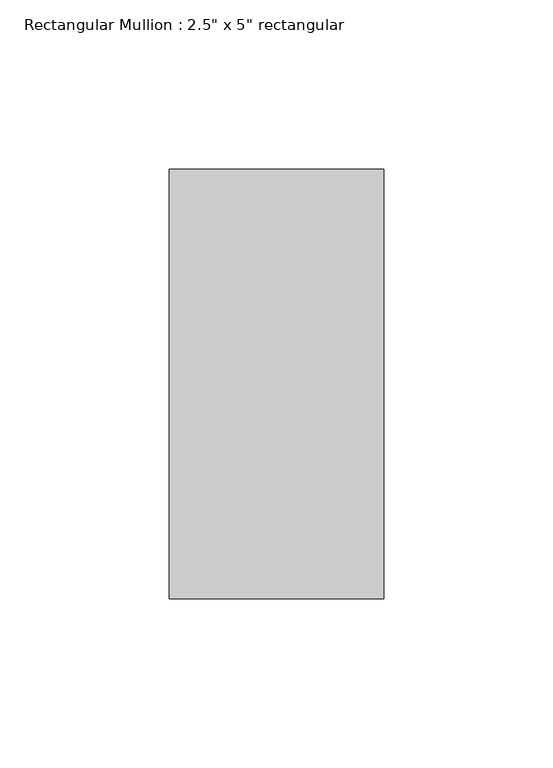
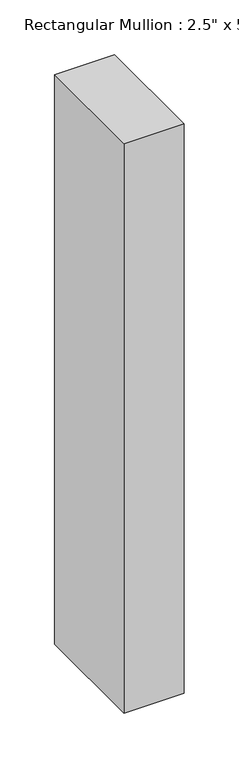
"""IFC4 building model written with IfcOpenShell, lengths in millimetres: member geometry."""

from ifc_helpers import new_model, si_unit, frame, origin, place, context, project, spatial, polyline, outline, extrude, source, transform, mapped, element, save


def member_5e365d0c(model_context):
    return source(origin(), model_context, "Body", "SweptSolid", [
        extrude(outline(polyline([(0.0, 63.5), (0.0, -63.5), (-63.5, -63.5), (-63.5, 63.5), (0.0, 63.5)])), frame((0.0, 0.0, -635.0), z_axis=(0.0, 0.0, 1.0), x_axis=(1.0, 0.0, 0.0)), (0.0, 0.0, 1.0), 635.0),
    ])


if __name__ == "__main__":
    model = new_model("IFC4")
    model_context = context("Model", 3, world=origin())
    ifc_project = project(units=[si_unit("LENGTHUNIT", "METRE", prefix="MILLI")], contexts=[model_context])
    site = spatial("IfcSite", under=ifc_project)
    building = spatial("IfcBuilding", under=site)
    placement = place(None, origin())
    member_shape = member_5e365d0c(model_context)
    element("IfcMember", 1, ObjectType="Rectangular Mullion : 2.5\" x 5\" rectangular", at=placement, inside=building, context=model_context, shape_type="MappedRepresentation", body=[
        mapped(member_shape, transform((0.0, 0.0, 0.0), x_axis=(1.0, 0.0, 0.0), y_axis=(0.0, 1.0, 0.0), z_axis=(0.0, 0.0, 1.0))),
    ])
    save(model, "model.ifc")

# Revit data of these elements
# Type "Rectangular Mullion : 2.5\" x 5\" rectangular"
#   built-in parameter 1007304 = 0.416667 (stored number, unit not read)
#   built-in parameter 1007301 = 0.104167 (stored number, unit not read)
#   built-in parameter 1007300 = 0.104167 (stored number, unit not read)
# Element 1 (IfcMember, "Rectangular Mullion : 2.5\" x 5\" rectangular")
#   Materials on its faces: "Aluminum"
# Materials
#   "Aluminum": class "Metal", colour RGB 247 247 247, transparency 0, Description = "Aluminum 6061", Cost = 0
